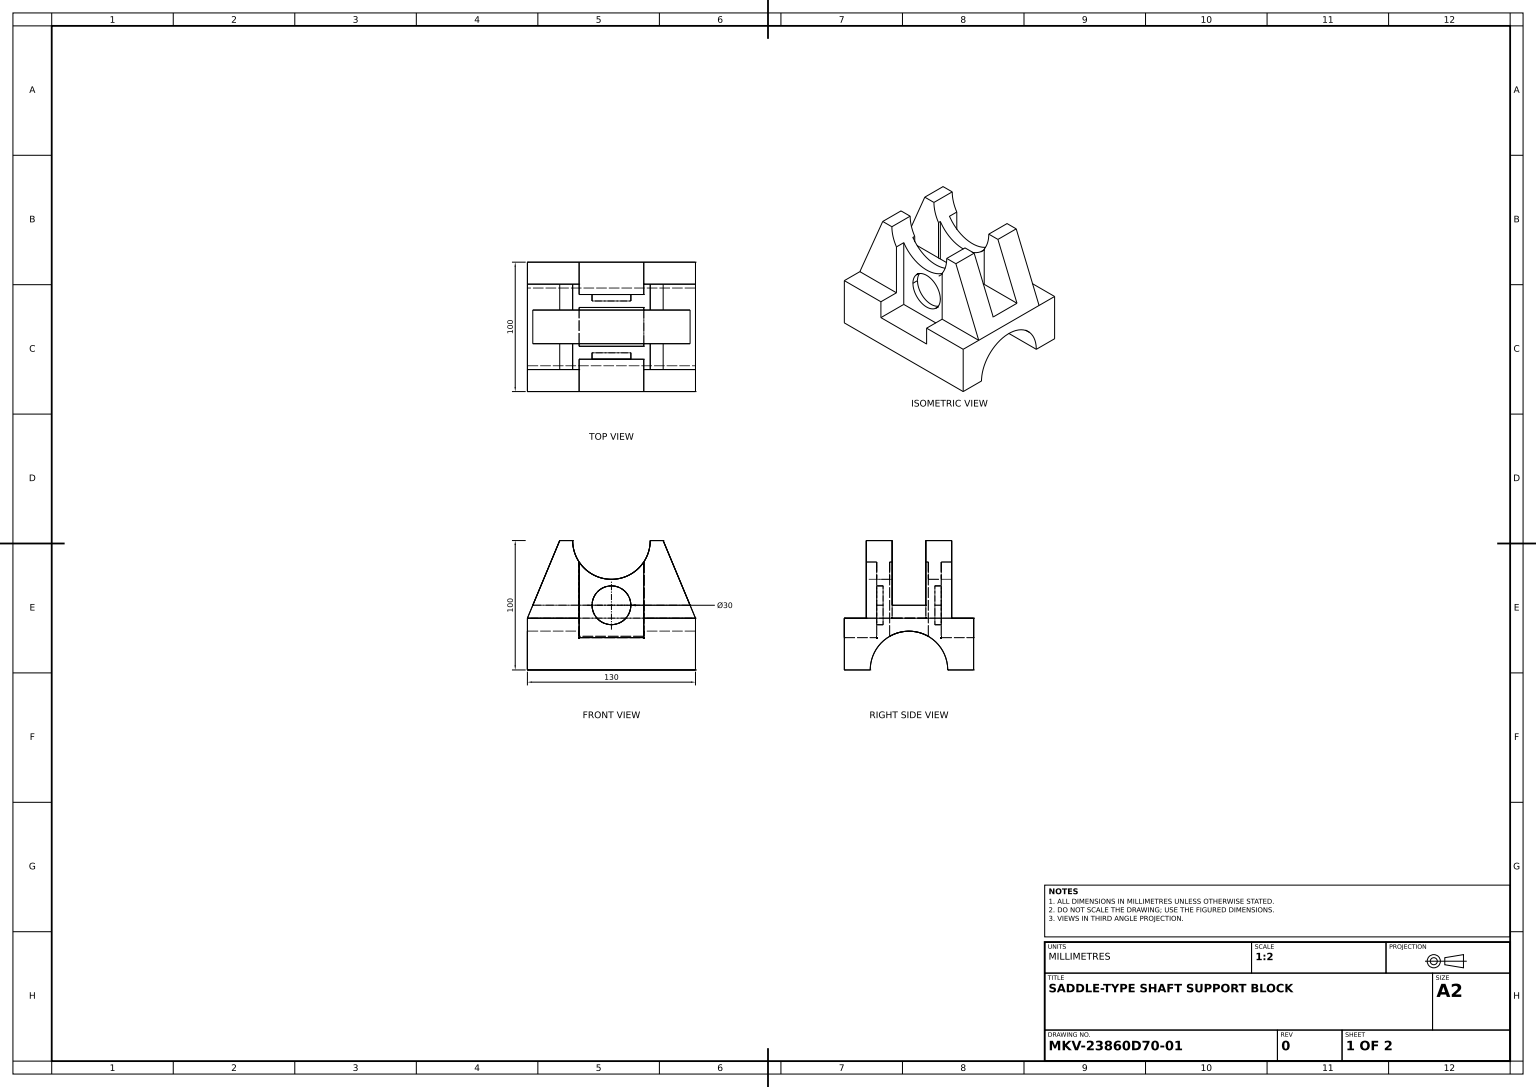
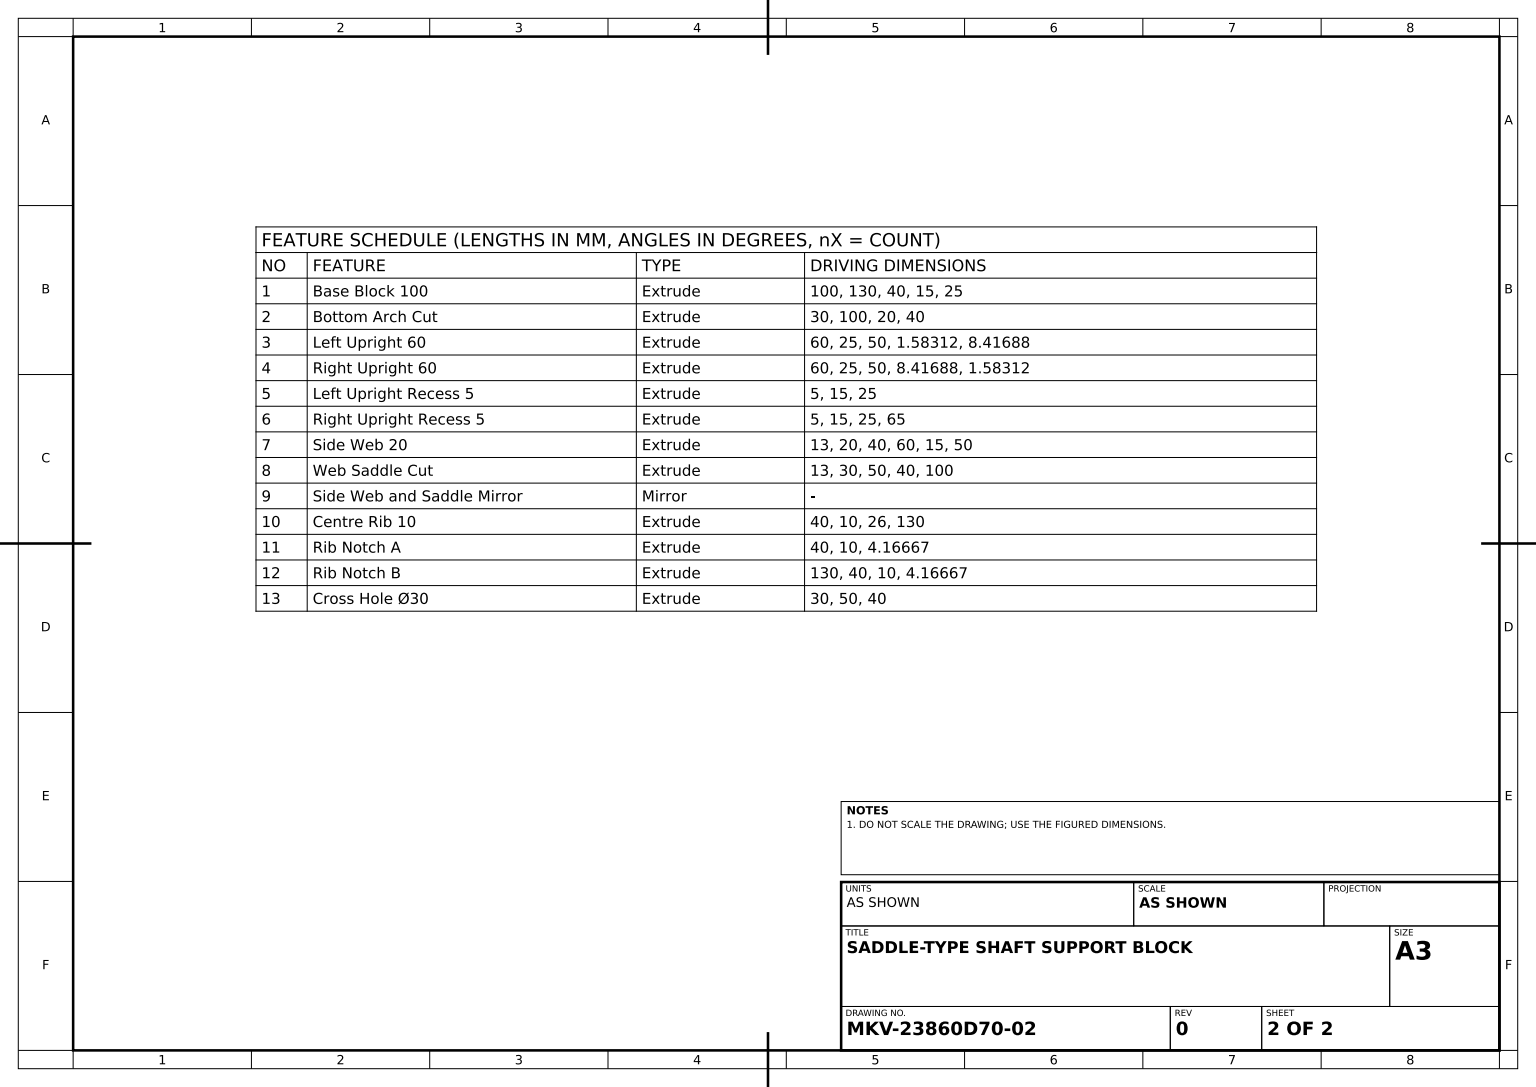
from build123d import *

# Parameters (mm, degrees)
BASE_BLOCK_100_DEPTH          = 50
BOTTOM_ARCH_CUT_DEPTH         = 145.913767462
LEFT_UPRIGHT_SKETCH_W         = 50
LEFT_UPRIGHT_SKETCH_H         = 1.583123952
LEFT_UPRIGHT_60_DEPTH         = 60
RIGHT_UPRIGHT_60_DEPTH        = 60
LEFT_UPRIGHT_RECESS_SKETCH_R  = 15
LEFT_UPRIGHT_RECESS_5_DEPTH   = 5
RIGHT_START                   = -5
RIGHT_UPRIGHT_RECESS_SKETCH_R = 15
RIGHT_UPRIGHT_RECESS_5_DEPTH  = 5
SIDE_WEB_20_DEPTH             = 20
WEB_SADDLE_SKETCH_R           = 30
WEB_SADDLE_CUT_DEPTH          = 176.695759767
CENTRE_RIB_SKETCH_W           = 130
CENTRE_RIB_SKETCH_H           = 26
CENTRE_RIB_10_DEPTH           = 10
RIB_NOTCH_A_DEPTH             = 176.695759767
RIB_NOTCH_B_DEPTH             = 176.695759767
CROSS_HOLE_SKETCH_R           = 30
CROSS_HOLE_30_DEPTH           = 172.464281995


with BuildPart() as part:
    # Base Profile Sketch → Base Block 100 (new, symmetric)
    with BuildSketch(Plane.XY):
        Polygon((0, 40), (0, 0), (130, 0), (130, 40), (90, 40), (90, 25), (65, 25), (40, 25), (40, 40), align=None)
    base_block_100 = extrude(amount=BASE_BLOCK_100_DEPTH, both=True)

    # Bottom Arch Sketch → Bottom Arch Cut (cut, through all)
    with BuildSketch(Plane(origin=(130, 0, 0), x_dir=(0, 0, -1), z_dir=(1, 0, 0))):
        with BuildLine():
            Line((-30, 0), (30, 0))
            ThreePointArc((30, 0), (0, 30), (-30, 0))
        make_face()
        with BuildLine():
            ThreePointArc((-30, 0), (0, -30), (30, 0))
            Line((30, 0), (-30, 0))
        make_face()
    extrude(amount=-BOTTOM_ARCH_CUT_DEPTH, mode=Mode.SUBTRACT)

    # Left Upright Sketch → Left Upright 60 (add)
    with BuildSketch(Plane(origin=(0, 25, 0), x_dir=(1, 0, 0), z_dir=(0, 1, 0))):
        with Locations((65, -15.791561976)):
            Rectangle(LEFT_UPRIGHT_SKETCH_W, LEFT_UPRIGHT_SKETCH_H)
        Polygon((40, -25), (65, -25), (90, -25), (90, -16.583123952), (40, -16.583123952), align=None)
    extrude(amount=LEFT_UPRIGHT_60_DEPTH)

    # Right Upright Sketch → Right Upright 60 (add)
    with BuildSketch(Plane(origin=(0, 25, 0), x_dir=(1, 0, 0), z_dir=(0, 1, 0))):
        Polygon((90, 25), (65, 25), (40, 25), (40, 15), (90, 15), align=None)
    extrude(amount=RIGHT_UPRIGHT_60_DEPTH)

    # Left Upright Recess Sketch → Left Upright Recess 5 (cut)
    with BuildSketch(Plane.XY.offset(25)):
        with Locations((65, 50)):
            Circle(LEFT_UPRIGHT_RECESS_SKETCH_R)
    extrude(amount=-LEFT_UPRIGHT_RECESS_5_DEPTH, mode=Mode.SUBTRACT)

    # Right Upright Recess Sketch → Right Upright Recess 5 (cut)
    with BuildSketch(Plane(origin=(0, 0, -25), x_dir=(-1, 0, 0), z_dir=(0, 0, -1)).offset(RIGHT_START)):
        with Locations(Location((-65, 50, 0), (0, 0, 180))):
            Circle(RIGHT_UPRIGHT_RECESS_SKETCH_R)
    extrude(amount=RIGHT_UPRIGHT_RECESS_5_DEPTH, mode=Mode.SUBTRACT)

    # Side Web Sketch → Side Web 20 (add)
    with BuildSketch(Plane.XY.offset(13)):
        Polygon((40, 40), (40, 100), (25, 100), (0, 40), align=None)
        Polygon((90, 40), (90, 100), (105, 100), (130, 40), align=None)
    side_web_20 = extrude(amount=SIDE_WEB_20_DEPTH)

    # Web Saddle Sketch → Web Saddle Cut (cut, symmetric)
    with BuildSketch(Plane.XY.offset(13)):
        with Locations((65, 100)):
            Circle(WEB_SADDLE_SKETCH_R)
    web_saddle_cut = extrude(amount=WEB_SADDLE_CUT_DEPTH, both=True, mode=Mode.SUBTRACT)

    # Side Web and Saddle Mirror: Base Block 100, Side Web 20, Web Saddle Cut across plane
    add(base_block_100.mirror(Plane.XY))
    add(side_web_20.mirror(Plane.XY))
    add(web_saddle_cut.mirror(Plane.XY), mode=Mode.SUBTRACT)

    # Centre Rib Sketch → Centre Rib 10 (add)
    with BuildSketch(Plane(origin=(0, 40, 0), x_dir=(1, 0, 0), z_dir=(0, 1, 0))):
        with Locations((65, 0)):
            Rectangle(CENTRE_RIB_SKETCH_W, CENTRE_RIB_SKETCH_H)
    extrude(amount=CENTRE_RIB_10_DEPTH)

    # Rib Notch A Sketch → Rib Notch A (cut, through all)
    with BuildSketch(Plane.XY.offset(13)):
        Polygon((4.166666667, 50), (0, 50), (0, 40), align=None)
    extrude(amount=-RIB_NOTCH_A_DEPTH, mode=Mode.SUBTRACT)

    # Rib Notch B Sketch → Rib Notch B (cut, through all)
    with BuildSketch(Plane.XY.offset(13)):
        Polygon((125.833333333, 50), (130, 40), (130, 50), align=None)
    extrude(amount=-RIB_NOTCH_B_DEPTH, mode=Mode.SUBTRACT)

    # Cross Hole Sketch → Cross Hole Ø30 (cut, through all)
    with BuildSketch(Plane(origin=(130, 0, 0), x_dir=(0, 0, -1), z_dir=(1, 0, 0))):
        Circle(CROSS_HOLE_SKETCH_R)
    extrude(amount=-CROSS_HOLE_30_DEPTH, mode=Mode.SUBTRACT)


solid = part.part
